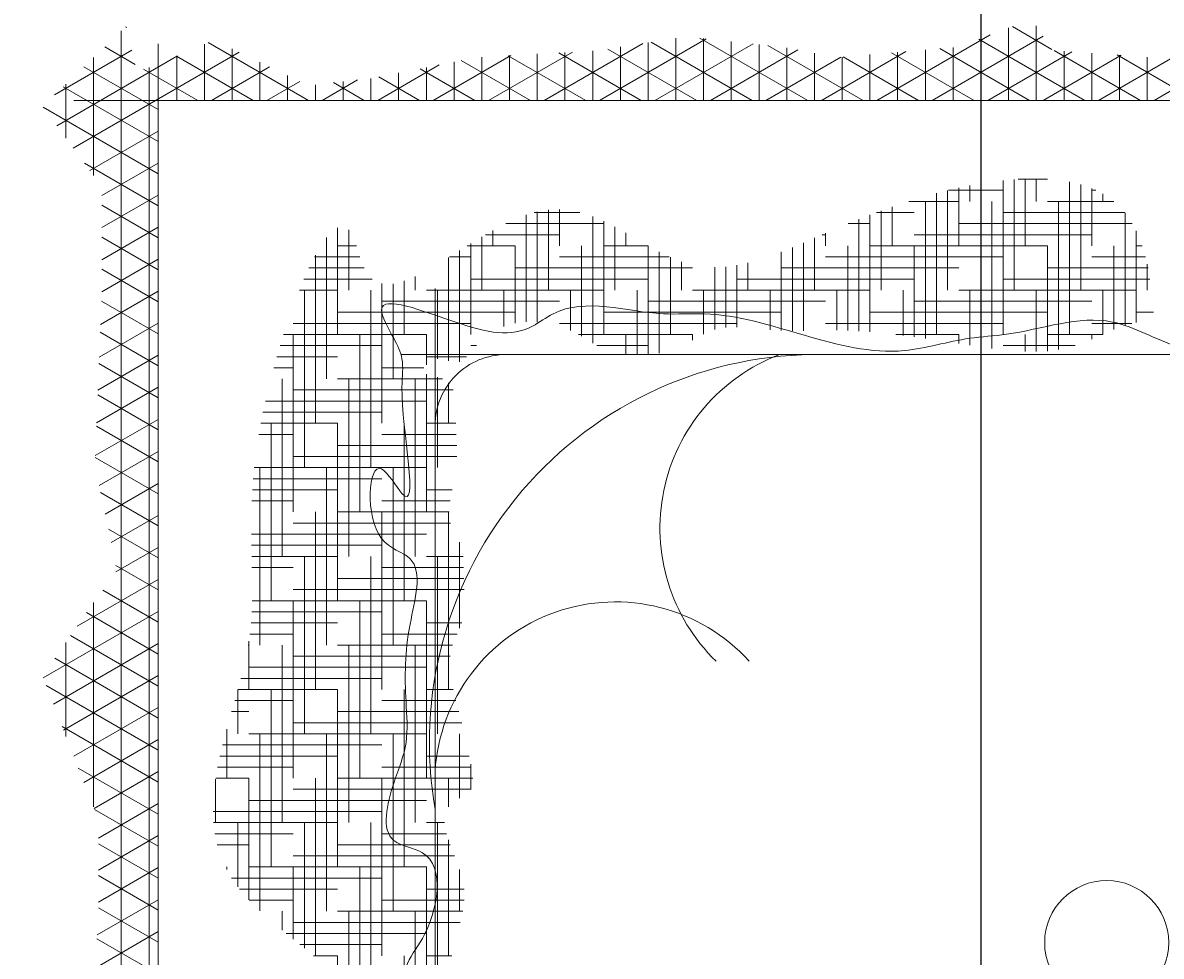
# Model space of a CAD drawing. Units: inches. Extents: x 3731 to 4318, y 1310 to 2388.
# Tile 12 of 57: x 3985 to 4038, y 1420 to 1463. Entities that reach past the tile are written whole.
import ezdxf

# ---------------------------------------------------------------- set-up
doc = ezdxf.new("R2010")
doc.units = ezdxf.units.IN
doc.layers.add('A-ANNO-DIMS', color=2, linetype='Continuous', lineweight=18)
doc.layers.add('A-FURN', color=8, linetype='Continuous', lineweight=13)
doc.styles.get("Standard").update_dxf_attribs({"font": 'arial.ttf'})
doc.dimstyles.get("Standard").update_dxf_attribs({"dimtxt": 0.18, "dimasz": 0.18, "dimexe": 0.18, "dimexo": 0.0625, "dimgap": 0.09, "dimtad": 0, "dimtih": 1, "dimtoh": 1, "dimdec": 4, "dimzin": 0, "dimdsep": 46, "dimtxsty": 'Standard', "dimcen": 0.09, "dimadec": 0, "dimazin": 0, "dimtfac": 1, "dimtdec": 4, "dimtofl": 0, "dimtmove": 0, "dimatfit": 3, "dimfxl": 1, "dimtolj": 1, "dimtzin": 0, "dimarcsym": 0})

# ---------------------------------------------------------------- blocks, each defined once
blk = doc.blocks.new('A$C200C7901')
for p, q in [((2.3121, 1.6596), (2.3121, 0.0201)), ((2, 0.2957), (2, 1.2957)), ((2.0224, 0.9977), (2.0224, 1.1977)), ((2.0224, 0.9977), (2.0224, 1.1977)), ((1.9974, 0.5977), (1.9974, 0.7977)), ((1.9974, 0.5977), (1.9974, 0.7977)), ((2.0724, 0.5977), (2.0724, 0.7977)), ((2.0724, 0.5977), (2.0724, 0.7977)), ((2.1474, 0.5977), (2.1474, 0.7977)), ((2.1474, 0.5977), (2.1474, 0.7977)), ((1.9849, 0.5477), (1.9849, 0.7477)), ((1.9849, 0.5477), (1.9849, 0.7477)), ((2.0599, 0.5477), (2.0599, 0.7477)), ((2.0599, 0.5477), (2.0599, 0.7477)), ((2.1349, 0.5477), (2.1349, 0.7477)), ((2.1349, 0.5477), (2.1349, 0.7477)), ((0.4061, 0.3703), (2.0386, 0.3703)), ((2.4073, 0.0839), (0.9625, 0.0839))]:
    blk.add_line(p, q)
at = {"linetype": 'ByBlock'}
for p, q in [((2.3224, 0.0468), (2.3224, 1.6627)), ((2.3224, 0.0468), (2.3224, 1.6627)), ((2.3537, 0.0056), (2.3537, 1.634)), ((2.3537, 0.0056), (2.3537, 1.634)), ((2.0349, 1.0477), (2.0349, 1.2477)), ((2.0349, 1.0477), (2.0349, 1.2477)), ((2.0099, 0.9477), (2.0099, 1.1477)), ((2.0099, 0.9477), (2.0099, 1.1477)), ((2.0849, 0.9477), (2.0849, 1.1477)), ((2.0849, 0.9477), (2.0849, 1.1477)), ((1.9974, 0.8977), (1.9974, 1.0977)), ((1.9974, 0.8977), (1.9974, 1.0977)), ((2.0724, 0.8977), (2.0724, 1.0977)), ((2.0724, 0.8977), (2.0724, 1.0977)), ((2.0974, 0.9977), (2.0974, 1.0909)), ((2.0974, 0.9977), (2.0974, 1.0909)), ((2.1099, 1.0477), (2.1099, 1.0729)), ((2.1099, 1.0477), (2.1099, 1.0729)), ((2.3121, 1.0686), (2.3813, 1.0286)), ((2.3121, 1.0686), (2.3813, 1.0286)), ((2.3121, 1.0206), (2.3851, 1.0628)), ((2.3121, 1.0206), (2.3851, 1.0628)), ((1.981, 1.0477), (2.0099, 1.0477)), ((1.981, 1.0477), (2.0099, 1.0477)), ((1.9849, 0.9171), (1.9849, 1.0477)), ((1.9849, 0.9171), (1.9849, 1.0477)), ((2.0599, 0.8477), (2.0599, 1.0477)), ((2.0599, 0.8477), (2.0599, 1.0477)), ((2.1099, 1.0477), (2.137, 1.0477)), ((2.1099, 1.0477), (2.137, 1.0477)), ((2.1349, 0.8477), (2.1349, 1.0477)), ((2.1349, 0.8477), (2.1349, 1.0477)), ((2.0599, 1.0352), (2.1523, 1.0352)), ((2.0599, 1.0352), (2.1523, 1.0352)), ((2.1474, 0.8977), (2.1474, 1.0391)), ((2.1474, 0.8977), (2.1474, 1.0391)), ((2.1599, 0.9477), (2.1599, 1.029)), ((2.1599, 0.9477), (2.1599, 1.029)), ((2.3121, 1.0325), (2.3795, 0.9936)), ((2.3121, 1.0325), (2.3795, 0.9936)), ((2.0099, 1.0227), (2.1678, 1.0227)), ((2.0099, 1.0227), (2.1678, 1.0227)), ((2.1724, 0.9977), (2.1724, 1.0189)), ((2.1724, 0.9977), (2.1724, 1.0189)), ((2.3121, 0.9846), (2.3809, 1.0242)), ((2.3121, 0.9846), (2.3809, 1.0242)), ((1.9718, 1.0102), (2.1599, 1.0102)), ((1.9718, 1.0102), (2.1599, 1.0102)), ((1.9688, 0.9977), (2.1099, 0.9977)), ((1.9688, 0.9977), (2.1099, 0.9977)), ((1.9724, 0.9504), (1.9724, 0.9977)), ((1.9724, 0.9504), (1.9724, 0.9977)), ((2.0474, 0.7977), (2.0474, 0.9977)), ((2.0474, 0.7977), (2.0474, 0.9977)), ((2.1224, 0.7977), (2.1224, 0.9977)), ((2.1224, 0.7977), (2.1224, 0.9977)), ((2.1974, 0.7977), (2.1974, 0.9972)), ((2.1974, 0.7977), (2.1974, 0.9972)), ((2.3121, 0.9964), (2.3795, 0.9575)), ((2.3121, 0.9964), (2.3795, 0.9575)), ((1.9671, 0.9852), (2.0599, 0.9852)), ((1.9671, 0.9852), (2.0599, 0.9852)), ((2.1599, 0.9852), (2.2095, 0.9852)), ((2.1599, 0.9852), (2.2095, 0.9852)), ((2.2099, 0.8477), (2.2099, 0.9848)), ((2.2099, 0.8477), (2.2099, 0.9848)), ((2.3121, 0.9485), (2.3795, 0.9874)), ((2.3121, 0.9485), (2.3795, 0.9874)), ((1.9672, 0.9727), (2.0099, 0.9727)), ((1.9672, 0.9727), (2.0099, 0.9727)), ((2.1099, 0.9727), (2.2204, 0.9727)), ((2.1099, 0.9727), (2.2204, 0.9727)), ((2.2224, 0.8977), (2.2224, 0.9702)), ((2.2224, 0.8977), (2.2224, 0.9702)), ((2.0599, 0.9602), (2.2294, 0.9602)), ((2.0599, 0.9602), (2.2294, 0.9602)), ((2.2349, 0.9477), (2.2349, 0.9506)), ((2.2349, 0.9477), (2.2349, 0.9506)), ((2.3121, 0.9603), (2.3795, 0.9215)), ((2.3121, 0.9603), (2.3795, 0.9215)), ((2.3121, 0.9124), (2.3795, 0.9513)), ((2.3121, 0.9124), (2.3795, 0.9513)), ((2.0099, 0.9477), (2.2099, 0.9477)), ((2.0099, 0.9477), (2.2099, 0.9477)), ((2.0349, 0.7477), (2.0349, 0.9477)), ((2.0349, 0.7477), (2.0349, 0.9477)), ((2.1099, 0.7477), (2.1099, 0.9477)), ((2.1099, 0.7477), (2.1099, 0.9477)), ((2.1849, 0.7477), (2.1849, 0.9477)), ((2.1849, 0.7477), (2.1849, 0.9477)), ((1.9781, 0.9352), (2.1599, 0.9352)), ((1.9781, 0.9352), (2.1599, 0.9352)), ((2.3121, 0.9243), (2.3838, 0.8829)), ((2.3121, 0.9243), (2.3838, 0.8829)), ((1.9829, 0.9227), (2.1099, 0.9227)), ((1.9829, 0.9227), (2.1099, 0.9227)), ((2.2099, 0.9227), (2.2455, 0.9227)), ((2.2099, 0.9227), (2.2455, 0.9227)), ((2.3121, 0.8763), (2.3795, 0.9152)), ((2.3121, 0.8763), (2.3795, 0.9152)), ((1.9871, 0.9102), (2.0599, 0.9102)), ((1.9871, 0.9102), (2.0599, 0.9102)), ((2.1599, 0.9102), (2.2481, 0.9102)), ((2.1599, 0.9102), (2.2481, 0.9102)), ((1.9894, 0.8977), (2.0099, 0.8977)), ((1.9894, 0.8977), (2.0099, 0.8977)), ((2.0224, 0.6977), (2.0224, 0.8977)), ((2.0224, 0.6977), (2.0224, 0.8977)), ((2.0974, 0.6977), (2.0974, 0.8977)), ((2.0974, 0.6977), (2.0974, 0.8977)), ((2.1099, 0.8977), (2.2496, 0.8977)), ((2.1099, 0.8977), (2.2496, 0.8977)), ((2.1724, 0.6977), (2.1724, 0.8977)), ((2.1724, 0.6977), (2.1724, 0.8977)), ((2.2474, 0.8489), (2.2474, 0.8977)), ((2.2474, 0.8489), (2.2474, 0.8977)), ((2.3121, 0.8882), (2.4022, 0.8362)), ((2.3121, 0.8882), (2.4022, 0.8362)), ((1.9849, 0.8477), (1.9849, 0.88)), ((1.9849, 0.8477), (1.9849, 0.88)), ((2.0099, 0.8727), (2.2099, 0.8727)), ((2.0099, 0.8727), (2.2099, 0.8727)), ((2.0599, 0.8852), (2.2501, 0.8852)), ((2.0599, 0.8852), (2.2501, 0.8852)), ((2.3121, 0.8402), (2.3842, 0.8818)), ((2.3121, 0.8402), (2.3842, 0.8818)), ((2.3849, 0.6497), (2.3849, 0.8801)), ((2.3849, 0.6497), (2.3849, 0.8801)), ((1.9599, 0.8317), (1.9599, 0.8604)), ((1.9599, 0.8317), (1.9599, 0.8604)), ((1.9599, 0.8602), (2.1599, 0.8602)), ((1.9599, 0.8602), (2.1599, 0.8602)), ((1.9724, 0.7977), (1.9724, 0.8703)), ((1.9724, 0.7977), (1.9724, 0.8703)), ((1.9574, 0.8477), (2.1099, 0.8477)), ((1.9574, 0.8477), (2.1099, 0.8477)), ((2.0099, 0.6477), (2.0099, 0.8477)), ((2.0099, 0.6477), (2.0099, 0.8477)), ((2.0849, 0.6477), (2.0849, 0.8477)), ((2.0849, 0.6477), (2.0849, 0.8477)), ((2.1599, 0.6477), (2.1599, 0.8477)), ((2.1599, 0.6477), (2.1599, 0.8477)), ((2.2099, 0.8477), (2.2472, 0.8477)), ((2.2099, 0.8477), (2.2472, 0.8477)), ((2.2349, 0.7923), (2.2349, 0.8477)), ((2.2349, 0.7923), (2.2349, 0.8477)), ((2.3121, 0.8041), (2.3958, 0.8524)), ((2.3121, 0.8041), (2.3958, 0.8524)), ((2.3121, 0.8521), (2.4205, 0.7895)), ((2.3121, 0.8521), (2.4205, 0.7895)), ((1.9593, 0.8352), (2.0599, 0.8352)), ((1.9593, 0.8352), (2.0599, 0.8352)), ((2.1599, 0.8352), (2.2451, 0.8352)), ((2.1599, 0.8352), (2.2451, 0.8352)), ((1.9615, 0.8227), (2.0099, 0.8227)), ((1.9615, 0.8227), (2.0099, 0.8227)), ((2.1099, 0.8227), (2.2425, 0.8227)), ((2.1099, 0.8227), (2.2425, 0.8227)), ((2.3121, 0.7681), (2.4073, 0.823)), ((2.3121, 0.7681), (2.4073, 0.823)), ((2.0599, 0.8102), (2.2396, 0.8102)), ((2.0599, 0.8102), (2.2396, 0.8102)), ((2.3121, 0.816), (2.4384, 0.7431)), ((2.3121, 0.816), (2.4384, 0.7431)), ((2.0099, 0.7977), (2.2099, 0.7977)), ((2.0099, 0.7977), (2.2099, 0.7977)), ((2.2224, 0.7483), (2.2224, 0.7977)), ((2.2224, 0.7483), (2.2224, 0.7977)), ((2.4162, 0.6946), (2.4162, 0.8006)), ((2.4162, 0.6946), (2.4162, 0.8006)), ((1.9699, 0.7852), (2.1599, 0.7852)), ((1.9699, 0.7852), (2.1599, 0.7852)), ((2.3121, 0.732), (2.4189, 0.7936)), ((2.3121, 0.732), (2.4189, 0.7936)), ((1.9734, 0.7727), (2.1099, 0.7727)), ((1.9734, 0.7727), (2.1099, 0.7727)), ((2.2099, 0.7727), (2.2294, 0.7727)), ((2.2099, 0.7727), (2.2294, 0.7727)), ((2.3121, 0.7799), (2.4287, 0.7126)), ((2.3121, 0.7799), (2.4287, 0.7126)), ((1.9767, 0.7602), (2.0599, 0.7602)), ((1.9767, 0.7602), (2.0599, 0.7602)), ((2.1599, 0.7602), (2.2258, 0.7602)), ((2.1599, 0.7602), (2.2258, 0.7602)), ((2.3121, 0.6959), (2.4303, 0.7641)), ((2.3121, 0.6959), (2.4303, 0.7641)), ((1.9797, 0.7477), (2.0099, 0.7477)), ((1.9797, 0.7477), (2.0099, 0.7477)), ((2.1099, 0.7477), (2.2222, 0.7477)), ((2.1099, 0.7477), (2.2222, 0.7477)), ((2.2099, 0.6933), (2.2099, 0.7477)), ((2.2099, 0.6933), (2.2099, 0.7477)), ((2.0599, 0.7352), (2.2188, 0.7352)), ((2.0599, 0.7352), (2.2188, 0.7352)), ((2.3121, 0.7438), (2.4108, 0.6869)), ((2.3121, 0.7438), (2.4108, 0.6869)), ((2.3121, 0.6598), (2.4417, 0.7346)), ((2.3121, 0.6598), (2.4417, 0.7346)), ((2.0099, 0.7227), (2.2099, 0.7227)), ((2.0099, 0.7227), (2.2099, 0.7227)), ((1.9831, 0.7102), (2.1599, 0.7102)), ((1.9831, 0.7102), (2.1599, 0.7102)), ((2.3121, 0.7078), (2.3929, 0.6611)), ((2.3121, 0.7078), (2.3929, 0.6611)), ((1.9804, 0.6977), (2.1099, 0.6977)), ((1.9804, 0.6977), (2.1099, 0.6977)), ((2.0474, 0.4977), (2.0474, 0.6977)), ((2.0474, 0.4977), (2.0474, 0.6977)), ((2.1224, 0.4977), (2.1224, 0.6977)), ((2.1224, 0.4977), (2.1224, 0.6977)), ((2.1974, 0.4977), (2.1974, 0.6977)), ((2.1974, 0.4977), (2.1974, 0.6977)), ((2.2099, 0.6977), (2.2106, 0.6977)), ((2.2099, 0.6977), (2.2106, 0.6977)), ((1.9753, 0.6852), (2.0599, 0.6852)), ((1.9753, 0.6852), (2.0599, 0.6852)), ((2.1599, 0.6852), (2.2088, 0.6852)), ((2.1599, 0.6852), (2.2088, 0.6852)), ((1.97, 0.6727), (2.0099, 0.6727)), ((1.97, 0.6727), (2.0099, 0.6727)), ((1.9724, 0.5818), (1.9724, 0.6786)), ((1.9724, 0.5818), (1.9724, 0.6786)), ((2.1099, 0.6727), (2.2075, 0.6727)), ((2.1099, 0.6727), (2.2075, 0.6727)), ((2.3121, 0.6237), (2.4036, 0.6765)), ((2.3121, 0.6237), (2.4036, 0.6765)), ((2.3121, 0.6717), (2.3744, 0.6357)), ((2.3121, 0.6717), (2.3744, 0.6357)), ((2.0599, 0.6602), (2.2067, 0.6602)), ((2.0599, 0.6602), (2.2067, 0.6602)), ((2.0099, 0.6477), (2.2062, 0.6477)), ((2.0099, 0.6477), (2.2062, 0.6477)), ((2.0349, 0.4477), (2.0349, 0.6477)), ((2.0349, 0.4477), (2.0349, 0.6477)), ((2.1099, 0.4477), (2.1099, 0.6477)), ((2.1099, 0.4477), (2.1099, 0.6477)), ((2.1849, 0.4477), (2.1849, 0.6477)), ((2.1849, 0.4477), (2.1849, 0.6477)), ((1.9673, 0.6352), (2.1599, 0.6352)), ((1.9673, 0.6352), (2.1599, 0.6352)), ((2.3121, 0.6356), (2.3598, 0.6081)), ((2.3121, 0.6356), (2.3598, 0.6081)), ((1.9678, 0.6227), (2.1099, 0.6227)), ((1.9678, 0.6227), (2.1099, 0.6227)), ((1.9679, 0.6102), (2.0599, 0.6102)), ((1.9679, 0.6102), (2.0599, 0.6102)), ((2.1599, 0.6102), (2.2064, 0.6102)), ((2.1599, 0.6102), (2.2064, 0.6102)), ((2.3121, 0.5876), (2.3598, 0.6151)), ((2.3121, 0.5876), (2.3598, 0.6151)), ((1.9685, 0.5977), (2.0099, 0.5977)), ((1.9685, 0.5977), (2.0099, 0.5977)), ((2.0224, 0.3977), (2.0224, 0.5977)), ((2.0224, 0.3977), (2.0224, 0.5977)), ((2.0974, 0.3977), (2.0974, 0.5977)), ((2.0974, 0.3977), (2.0974, 0.5977)), ((2.1099, 0.5977), (2.2066, 0.5977)), ((2.1099, 0.5977), (2.2066, 0.5977)), ((2.1724, 0.3977), (2.1724, 0.5977)), ((2.1724, 0.3977), (2.1724, 0.5977)), ((2.3121, 0.5995), (2.3682, 0.5671)), ((2.3121, 0.5995), (2.3682, 0.5671)), ((2.0599, 0.5852), (2.2069, 0.5852)), ((2.0599, 0.5852), (2.2069, 0.5852)), ((2.3121, 0.5515), (2.365, 0.5821)), ((2.3121, 0.5515), (2.365, 0.5821)), ((2.0099, 0.5727), (2.207, 0.5727)), ((2.0099, 0.5727), (2.207, 0.5727)), ((1.9827, 0.5602), (2.1599, 0.5602)), ((1.9827, 0.5602), (2.1599, 0.5602)), ((2.3121, 0.5634), (2.3771, 0.5259)), ((2.3121, 0.5634), (2.3771, 0.5259)), ((1.9842, 0.5477), (2.1099, 0.5477)), ((1.9842, 0.5477), (2.1099, 0.5477)), ((2.0099, 0.3923), (2.0099, 0.5477)), ((2.0099, 0.3923), (2.0099, 0.5477)), ((2.0849, 0.3477), (2.0849, 0.5477)), ((2.0849, 0.3477), (2.0849, 0.5477)), ((2.1599, 0.3477), (2.1599, 0.5477)), ((2.1599, 0.3477), (2.1599, 0.5477)), ((2.3121, 0.5155), (2.3719, 0.55)), ((2.3121, 0.5155), (2.3719, 0.55)), ((1.9831, 0.5352), (2.0599, 0.5352)), ((1.9831, 0.5352), (2.0599, 0.5352)), ((2.1599, 0.5352), (2.2065, 0.5352)), ((2.1599, 0.5352), (2.2065, 0.5352)), ((2.3121, 0.5273), (2.383, 0.4864)), ((2.3121, 0.5273), (2.383, 0.4864)), ((1.9807, 0.5227), (2.0099, 0.5227)), ((1.9807, 0.5227), (2.0099, 0.5227)), ((2.1099, 0.5227), (2.2058, 0.5227)), ((2.1099, 0.5227), (2.2058, 0.5227)), ((2.3121, 0.4794), (2.3788, 0.5179)), ((2.3121, 0.4794), (2.3788, 0.5179)), ((2.0599, 0.5102), (2.2049, 0.5102)), ((2.0599, 0.5102), (2.2049, 0.5102)), ((1.9974, 0.3957), (1.9974, 0.4977)), ((1.9974, 0.3957), (1.9974, 0.4977)), ((2.0099, 0.4977), (2.2038, 0.4977)), ((2.0099, 0.4977), (2.2038, 0.4977)), ((2.0724, 0.2977), (2.0724, 0.4977)), ((2.0724, 0.2977), (2.0724, 0.4977)), ((2.1474, 0.2977), (2.1474, 0.4977)), ((2.1474, 0.2977), (2.1474, 0.4977)), ((2.3121, 0.4912), (2.3817, 0.4511)), ((2.3121, 0.4912), (2.3817, 0.4511)), ((1.9755, 0.4852), (2.1599, 0.4852)), ((1.9755, 0.4852), (2.1599, 0.4852)), ((2.3121, 0.4433), (2.383, 0.4842)), ((2.3121, 0.4433), (2.383, 0.4842)), ((1.9757, 0.4727), (2.1099, 0.4727)), ((1.9757, 0.4727), (2.1099, 0.4727)), ((1.9762, 0.4602), (2.0599, 0.4602)), ((1.9762, 0.4602), (2.0599, 0.4602)), ((2.1599, 0.4602), (2.1987, 0.4602)), ((2.1599, 0.4602), (2.1987, 0.4602)), ((2.3121, 0.4552), (2.3803, 0.4158)), ((2.3121, 0.4552), (2.3803, 0.4158)), ((1.9768, 0.4477), (2.0099, 0.4477)), ((1.9768, 0.4477), (2.0099, 0.4477)), ((1.9849, 0.402), (1.9849, 0.4477)), ((1.9849, 0.402), (1.9849, 0.4477)), ((2.0599, 0.2903), (2.0599, 0.4477)), ((2.0599, 0.2903), (2.0599, 0.4477)), ((2.1099, 0.4477), (2.1965, 0.4477)), ((2.1099, 0.4477), (2.1965, 0.4477)), ((2.1349, 0.2582), (2.1349, 0.4477)), ((2.1349, 0.2582), (2.1349, 0.4477)), ((2.3121, 0.4072), (2.3815, 0.4473)), ((2.3121, 0.4072), (2.3815, 0.4473)), ((2.0599, 0.4352), (2.194, 0.4352)), ((2.0599, 0.4352), (2.194, 0.4352)), ((2.0099, 0.4227), (2.1913, 0.4227)), ((2.0099, 0.4227), (2.1913, 0.4227)), ((2.3121, 0.4191), (2.3789, 0.3805)), ((2.3121, 0.4191), (2.3789, 0.3805)), ((1.9797, 0.4102), (2.1599, 0.4102)), ((1.9797, 0.4102), (2.1599, 0.4102)), ((2.3121, 0.3711), (2.3801, 0.4103)), ((2.3121, 0.3711), (2.3801, 0.4103)), ((1.9915, 0.3977), (2.1099, 0.3977)), ((1.9915, 0.3977), (2.1099, 0.3977)), ((2.0127, 0.3852), (2.0599, 0.3852)), ((2.0127, 0.3852), (2.0599, 0.3852)), ((2.0474, 0.2905), (2.0474, 0.3977)), ((2.0474, 0.2905), (2.0474, 0.3977)), ((2.1224, 0.2385), (2.1224, 0.3977)), ((2.1224, 0.2385), (2.1224, 0.3977)), ((2.1599, 0.3852), (2.1819, 0.3852)), ((2.1599, 0.3852), (2.1819, 0.3852)), ((1.9648, 0.3727), (2.0099, 0.3727)), ((1.9648, 0.3727), (2.0099, 0.3727)), ((1.9724, 0.253), (1.9724, 0.3785)), ((1.9724, 0.253), (1.9724, 0.3785)), ((1.9849, 0.2609), (1.9849, 0.3774)), ((1.9849, 0.2609), (1.9849, 0.3774)), ((1.9974, 0.2977), (1.9974, 0.3753)), ((1.9974, 0.2977), (1.9974, 0.3753)), ((2.0099, 0.3477), (2.0099, 0.382)), ((2.0099, 0.3477), (2.0099, 0.382)), ((2.1099, 0.3727), (2.1784, 0.3727)), ((2.1099, 0.3727), (2.1784, 0.3727)), ((2.3121, 0.383), (2.3775, 0.3452)), ((2.3121, 0.383), (2.3775, 0.3452)), ((2.3121, 0.335), (2.3786, 0.3734)), ((2.3121, 0.335), (2.3786, 0.3734)), ((1.2785, 0.3602), (1.3599, 0.3602)), ((1.2785, 0.3602), (1.3599, 0.3602)), ((1.2974, 0.1977), (1.2974, 0.3647)), ((1.2974, 0.1977), (1.2974, 0.3647)), ((1.3099, 0.2477), (1.3099, 0.3663)), ((1.3099, 0.2477), (1.3099, 0.3663)), ((1.3224, 0.2977), (1.3224, 0.3669)), ((1.3224, 0.2977), (1.3224, 0.3669)), ((1.3349, 0.3477), (1.3349, 0.3668)), ((1.3349, 0.3477), (1.3349, 0.3668)), ((1.3724, 0.1977), (1.3724, 0.3634)), ((1.3724, 0.1977), (1.3724, 0.3634)), ((1.3849, 0.2477), (1.3849, 0.3616)), ((1.3849, 0.2477), (1.3849, 0.3616)), ((1.3974, 0.2977), (1.3974, 0.3597)), ((1.3974, 0.2977), (1.3974, 0.3597)), ((1.7474, 0.2546), (1.7474, 0.3689)), ((1.7474, 0.2546), (1.7474, 0.3689)), ((1.7599, 0.2477), (1.7599, 0.3703)), ((1.7599, 0.2477), (1.7599, 0.3703)), ((1.7599, 0.3602), (1.8177, 0.3602)), ((1.7599, 0.3602), (1.8177, 0.3602)), ((1.7724, 0.2977), (1.7724, 0.3703)), ((1.7724, 0.2977), (1.7724, 0.3703)), ((1.7849, 0.3477), (1.7849, 0.3703)), ((1.7849, 0.3477), (1.7849, 0.3703)), ((1.9532, 0.3602), (1.9599, 0.3602)), ((1.9532, 0.3602), (1.9599, 0.3602)), ((2.0599, 0.3602), (2.1747, 0.3602)), ((2.0599, 0.3602), (2.1747, 0.3602)), ((1.2474, 0.2977), (1.2474, 0.3476)), ((1.2474, 0.2977), (1.2474, 0.3476)), ((1.2475, 0.3477), (1.3099, 0.3477)), ((1.2475, 0.3477), (1.3099, 0.3477)), ((1.2599, 0.3477), (1.2599, 0.3531)), ((1.2599, 0.3477), (1.2599, 0.3531)), ((1.2849, 0.1758), (1.2849, 0.3477)), ((1.2849, 0.1758), (1.2849, 0.3477)), ((1.3599, 0.1741), (1.3599, 0.3477)), ((1.3599, 0.1741), (1.3599, 0.3477)), ((1.4099, 0.3477), (1.4099, 0.3578)), ((1.4099, 0.3477), (1.4099, 0.3578)), ((1.4099, 0.3477), (1.4806, 0.3477)), ((1.4099, 0.3477), (1.4806, 0.3477)), ((1.4349, 0.1886), (1.4349, 0.3477)), ((1.4349, 0.1886), (1.4349, 0.3477)), ((1.4474, 0.1977), (1.4474, 0.3521)), ((1.4474, 0.1977), (1.4474, 0.3521)), ((1.4599, 0.2477), (1.4599, 0.3504)), ((1.4599, 0.2477), (1.4599, 0.3504)), ((1.4724, 0.2977), (1.4724, 0.3487)), ((1.4724, 0.2977), (1.4724, 0.3487)), ((1.6974, 0.2977), (1.6974, 0.3472)), ((1.6974, 0.2977), (1.6974, 0.3472)), ((1.7099, 0.3477), (1.7099, 0.3539)), ((1.7099, 0.3477), (1.7099, 0.3539)), ((1.7099, 0.3477), (1.8383, 0.3477)), ((1.7099, 0.3477), (1.8383, 0.3477)), ((1.7349, 0.2607), (1.7349, 0.3477)), ((1.7349, 0.2607), (1.7349, 0.3477)), ((1.8099, 0.2201), (1.8099, 0.3477)), ((1.8099, 0.2201), (1.8099, 0.3477)), ((1.8224, 0.2148), (1.8224, 0.3575)), ((1.8224, 0.2148), (1.8224, 0.3575)), ((1.8349, 0.2477), (1.8349, 0.3497)), ((1.8349, 0.2477), (1.8349, 0.3497)), ((1.9599, 0.2452), (1.9599, 0.3477)), ((1.9599, 0.2452), (1.9599, 0.3477)), ((2.0099, 0.3477), (2.1708, 0.3477)), ((2.0099, 0.3477), (2.1708, 0.3477)), ((2.0349, 0.2874), (2.0349, 0.3477)), ((2.0349, 0.2874), (2.0349, 0.3477)), ((2.1099, 0.2274), (2.1099, 0.3477)), ((2.1099, 0.2274), (2.1099, 0.3477)), ((2.3121, 0.3469), (2.3761, 0.31)), ((2.3121, 0.3469), (2.3761, 0.31)), ((1.2099, 0.2308), (1.2099, 0.334)), ((1.2099, 0.2308), (1.2099, 0.334)), ((1.2148, 0.3352), (1.2599, 0.3352)), ((1.2148, 0.3352), (1.2599, 0.3352)), ((1.2224, 0.2106), (1.2224, 0.3375)), ((1.2224, 0.2106), (1.2224, 0.3375)), ((1.2349, 0.2477), (1.2349, 0.3422)), ((1.2349, 0.2477), (1.2349, 0.3422)), ((1.3599, 0.3352), (1.5599, 0.3352)), ((1.3599, 0.3352), (1.5599, 0.3352)), ((1.5099, 0.2129), (1.5099, 0.3447)), ((1.5099, 0.2129), (1.5099, 0.3447)), ((1.5224, 0.2177), (1.5224, 0.3438)), ((1.5224, 0.2177), (1.5224, 0.3438)), ((1.5349, 0.2477), (1.5349, 0.3431)), ((1.5349, 0.2477), (1.5349, 0.3431)), ((1.5474, 0.2977), (1.5474, 0.3428)), ((1.5474, 0.2977), (1.5474, 0.3428)), ((1.5849, 0.2443), (1.5849, 0.3434)), ((1.5849, 0.2443), (1.5849, 0.3434)), ((1.5974, 0.2496), (1.5974, 0.3435)), ((1.5974, 0.2496), (1.5974, 0.3435)), ((1.6099, 0.2546), (1.6099, 0.3432)), ((1.6099, 0.2546), (1.6099, 0.3432)), ((1.6224, 0.2977), (1.6224, 0.3424)), ((1.6224, 0.2977), (1.6224, 0.3424)), ((1.6599, 0.2695), (1.6599, 0.3394)), ((1.6599, 0.2695), (1.6599, 0.3394)), ((1.6599, 0.3352), (1.8599, 0.3352)), ((1.6599, 0.3352), (1.8599, 0.3352)), ((1.6724, 0.2713), (1.6724, 0.3398)), ((1.6724, 0.2713), (1.6724, 0.3398)), ((1.6849, 0.272), (1.6849, 0.3422)), ((1.6849, 0.272), (1.6849, 0.3422)), ((1.8474, 0.2977), (1.8474, 0.3432)), ((1.8474, 0.2977), (1.8474, 0.3432)), ((1.8849, 0.2093), (1.8849, 0.3337)), ((1.8849, 0.2093), (1.8849, 0.3337)), ((1.9099, 0.2477), (1.9099, 0.3349)), ((1.9099, 0.2477), (1.9099, 0.3349)), ((1.9224, 0.2977), (1.9224, 0.3385)), ((1.9224, 0.2977), (1.9224, 0.3385)), ((1.9599, 0.3352), (2.1599, 0.3352)), ((1.9599, 0.3352), (2.1599, 0.3352)), ((2.3121, 0.299), (2.3772, 0.3365)), ((2.3121, 0.299), (2.3772, 0.3365)), ((1.1904, 0.3227), (1.2099, 0.3227)), ((1.1904, 0.3227), (1.2099, 0.3227)), ((1.3099, 0.3227), (1.5099, 0.3227)), ((1.3099, 0.3227), (1.5099, 0.3227)), ((1.6099, 0.3227), (1.8099, 0.3227)), ((1.6099, 0.3227), (1.8099, 0.3227)), ((1.8974, 0.2129), (1.8974, 0.3335)), ((1.8974, 0.2129), (1.8974, 0.3335)), ((1.9099, 0.3227), (2.1099, 0.3227)), ((1.9099, 0.3227), (2.1099, 0.3227)), ((1.2599, 0.3102), (1.4599, 0.3102)), ((1.2599, 0.3102), (1.4599, 0.3102)), ((1.5599, 0.3102), (1.7599, 0.3102)), ((1.5599, 0.3102), (1.7599, 0.3102)), ((1.8599, 0.3102), (2.0599, 0.3102)), ((1.8599, 0.3102), (2.0599, 0.3102)), ((2.3121, 0.3108), (2.3755, 0.2742)), ((2.3121, 0.3108), (2.3755, 0.2742)), ((1.1974, 0.2683), (1.1974, 0.2977)), ((1.1974, 0.2683), (1.1974, 0.2977)), ((1.2099, 0.2977), (1.4099, 0.2977)), ((1.2099, 0.2977), (1.4099, 0.2977)), ((1.2724, 0.1788), (1.2724, 0.2977)), ((1.2724, 0.1788), (1.2724, 0.2977)), ((1.3474, 0.173), (1.3474, 0.2977)), ((1.3474, 0.173), (1.3474, 0.2977)), ((1.4224, 0.1854), (1.4224, 0.2977)), ((1.4224, 0.1854), (1.4224, 0.2977)), ((1.4974, 0.2083), (1.4974, 0.2977)), ((1.4974, 0.2083), (1.4974, 0.2977)), ((1.5099, 0.2977), (1.7099, 0.2977)), ((1.5099, 0.2977), (1.7099, 0.2977)), ((1.5724, 0.2389), (1.5724, 0.2977)), ((1.5724, 0.2389), (1.5724, 0.2977)), ((1.6474, 0.2668), (1.6474, 0.2977)), ((1.6474, 0.2668), (1.6474, 0.2977)), ((1.7224, 0.2658), (1.7224, 0.2977)), ((1.7224, 0.2658), (1.7224, 0.2977)), ((1.7974, 0.2263), (1.7974, 0.2977)), ((1.7974, 0.2263), (1.7974, 0.2977)), ((1.8099, 0.2977), (2.0099, 0.2977)), ((1.8099, 0.2977), (2.0099, 0.2977)), ((1.8724, 0.2072), (1.8724, 0.2977)), ((1.8724, 0.2072), (1.8724, 0.2977)), ((1.9474, 0.2376), (1.9474, 0.2977)), ((1.9474, 0.2376), (1.9474, 0.2977)), ((2.0224, 0.2822), (2.0224, 0.2977)), ((2.0224, 0.2822), (2.0224, 0.2977)), ((2.0974, 0.2299), (2.0974, 0.2977)), ((2.0974, 0.2299), (2.0974, 0.2977)), ((2.1099, 0.2977), (2.153, 0.2977)), ((2.1099, 0.2977), (2.153, 0.2977)), ((2.3121, 0.2629), (2.3757, 0.2996)), ((2.3121, 0.2629), (2.3757, 0.2996)), ((1.1943, 0.2852), (1.3599, 0.2852)), ((1.1943, 0.2852), (1.3599, 0.2852)), ((1.4599, 0.2852), (1.6599, 0.2852)), ((1.4599, 0.2852), (1.6599, 0.2852)), ((1.7599, 0.2852), (1.9599, 0.2852)), ((1.7599, 0.2852), (1.9599, 0.2852)), ((2.0708, 0.2852), (2.1478, 0.2852)), ((2.0708, 0.2852), (2.1478, 0.2852)), ((1.1965, 0.2727), (1.3099, 0.2727)), ((1.1965, 0.2727), (1.3099, 0.2727)), ((1.4099, 0.2727), (1.6099, 0.2727)), ((1.4099, 0.2727), (1.6099, 0.2727)), ((1.7099, 0.2727), (1.9099, 0.2727)), ((1.7099, 0.2727), (1.9099, 0.2727)), ((2.08, 0.2727), (2.1422, 0.2727)), ((2.08, 0.2727), (2.1422, 0.2727)), ((2.3121, 0.2747), (2.3755, 0.2381)), ((2.3121, 0.2747), (2.3755, 0.2381)), ((1.1994, 0.2602), (1.2599, 0.2602)), ((1.1994, 0.2602), (1.2599, 0.2602)), ((1.3599, 0.2602), (1.5599, 0.2602)), ((1.3599, 0.2602), (1.5599, 0.2602)), ((1.7361, 0.2602), (1.8599, 0.2602)), ((1.7361, 0.2602), (1.8599, 0.2602)), ((1.9599, 0.2602), (1.9838, 0.2602)), ((1.9599, 0.2602), (1.9838, 0.2602)), ((2.0848, 0.2602), (2.1359, 0.2602)), ((2.0848, 0.2602), (2.1359, 0.2602)), ((2.3121, 0.2268), (2.3755, 0.2634)), ((2.3121, 0.2268), (2.3755, 0.2634)), ((1.2031, 0.2477), (1.2099, 0.2477)), ((1.2031, 0.2477), (1.2099, 0.2477)), ((1.2599, 0.1831), (1.2599, 0.2477)), ((1.2599, 0.1831), (1.2599, 0.2477)), ((1.3099, 0.2477), (1.5099, 0.2477)), ((1.3099, 0.2477), (1.5099, 0.2477)), ((1.3349, 0.1723), (1.3349, 0.2477)), ((1.3349, 0.1723), (1.3349, 0.2477)), ((1.4099, 0.1825), (1.4099, 0.2477)), ((1.4099, 0.1825), (1.4099, 0.2477)), ((1.4849, 0.2039), (1.4849, 0.2477)), ((1.4849, 0.2039), (1.4849, 0.2477)), ((1.5599, 0.2335), (1.5599, 0.2477)), ((1.5599, 0.2335), (1.5599, 0.2477)), ((1.7599, 0.2477), (1.8099, 0.2477)), ((1.7599, 0.2477), (1.8099, 0.2477)), ((1.7849, 0.2332), (1.7849, 0.2477)), ((1.7849, 0.2332), (1.7849, 0.2477)), ((1.8599, 0.2068), (1.8599, 0.2477)), ((1.8599, 0.2068), (1.8599, 0.2477)), ((1.9099, 0.2477), (1.9639, 0.2477)), ((1.9099, 0.2477), (1.9639, 0.2477)), ((1.9349, 0.2304), (1.9349, 0.2477)), ((1.9349, 0.2304), (1.9349, 0.2477)), ((2.0888, 0.2477), (2.1099, 0.2477)), ((2.0888, 0.2477), (2.1099, 0.2477)), ((1.2599, 0.2352), (1.4599, 0.2352)), ((1.2599, 0.2352), (1.4599, 0.2352)), ((1.5599, 0.2352), (1.5638, 0.2352)), ((1.5599, 0.2352), (1.5638, 0.2352)), ((1.8599, 0.2352), (1.9433, 0.2352)), ((1.8599, 0.2352), (1.9433, 0.2352)), ((2.3121, 0.2387), (2.3755, 0.202)), ((2.3121, 0.2387), (2.3755, 0.202)), ((1.2142, 0.2227), (1.4099, 0.2227)), ((1.2142, 0.2227), (1.4099, 0.2227)), ((1.5099, 0.2227), (1.5346, 0.2227)), ((1.5099, 0.2227), (1.5346, 0.2227)), ((1.8099, 0.2227), (1.9203, 0.2227)), ((1.8099, 0.2227), (1.9203, 0.2227)), ((2.3121, 0.1907), (2.3755, 0.2273)), ((2.3121, 0.1907), (2.3755, 0.2273)), ((1.2227, 0.2102), (1.3599, 0.2102)), ((1.2227, 0.2102), (1.3599, 0.2102)), ((1.4599, 0.2102), (1.5027, 0.2102)), ((1.4599, 0.2102), (1.5027, 0.2102)), ((1.8368, 0.2102), (1.8884, 0.2102)), ((1.8368, 0.2102), (1.8884, 0.2102)), ((1.2351, 0.1977), (1.3099, 0.1977)), ((1.2351, 0.1977), (1.3099, 0.1977)), ((1.2474, 0.1892), (1.2474, 0.1977)), ((1.2474, 0.1892), (1.2474, 0.1977)), ((1.3224, 0.1722), (1.3224, 0.1977)), ((1.3224, 0.1722), (1.3224, 0.1977)), ((1.3974, 0.1799), (1.3974, 0.1977)), ((1.3974, 0.1799), (1.3974, 0.1977)), ((1.4099, 0.1977), (1.4662, 0.1977)), ((1.4099, 0.1977), (1.4662, 0.1977)), ((2.3121, 0.2026), (2.3953, 0.1545)), ((2.3121, 0.2026), (2.3953, 0.1545)), ((1.2552, 0.1852), (1.2599, 0.1852)), ((1.2552, 0.1852), (1.2599, 0.1852)), ((1.3599, 0.1852), (1.4215, 0.1852)), ((1.3599, 0.1852), (1.4215, 0.1852)), ((2.3121, 0.1546), (2.3755, 0.1912)), ((2.3121, 0.1546), (2.3755, 0.1912)), ((1.3099, 0.1727), (1.3428, 0.1727)), ((1.3099, 0.1727), (1.3428, 0.1727)), ((2.3849, 0.0355), (2.3849, 0.1686)), ((2.3849, 0.0355), (2.3849, 0.1686)), ((2.3121, 0.1665), (2.4419, 0.0916)), ((2.3121, 0.1665), (2.4419, 0.0916)), ((2.3121, 0.1185), (2.3891, 0.163)), ((2.3121, 0.1185), (2.3891, 0.163)), ((2.2208, 0.0297), (2.4078, 0.1377)), ((2.2208, 0.0297), (2.4078, 0.1377)), ((2.3121, 0.1304), (2.4193, 0.0685)), ((2.3121, 0.1304), (2.4193, 0.0685)), ((2.4162, 0.0655), (2.4162, 0.1264)), ((2.4162, 0.0655), (2.4162, 0.1264)), ((2.2903, 0.0337), (2.4265, 0.1124)), ((2.2903, 0.0337), (2.4265, 0.1124)), ((2.3121, 0.0943), (2.3958, 0.046)), ((2.3121, 0.0943), (2.3958, 0.046)), ((1.0891, 0.0259), (1.1897, 0.0839)), ((1.0891, 0.0259), (1.1897, 0.0839)), ((1.1426, 0.0839), (1.2313, 0.0327)), ((1.1426, 0.0839), (1.2313, 0.0327)), ((1.1642, 0.0331), (1.2522, 0.0839)), ((1.1642, 0.0331), (1.2522, 0.0839)), ((1.1974, 0.0351), (1.1974, 0.0839)), ((1.1974, 0.0351), (1.1974, 0.0839)), ((1.2051, 0.0839), (1.3023, 0.0278)), ((1.2051, 0.0839), (1.3023, 0.0278)), ((1.2266, 0.033), (1.3147, 0.0839)), ((1.2266, 0.033), (1.3147, 0.0839)), ((1.2287, 0.0329), (1.2287, 0.0839)), ((1.2287, 0.0329), (1.2287, 0.0839)), ((1.2599, 0.0308), (1.2599, 0.0839)), ((1.2599, 0.0308), (1.2599, 0.0839)), ((1.2676, 0.0839), (1.3871, 0.015)), ((1.2676, 0.0839), (1.3871, 0.015)), ((1.2824, 0.0292), (1.3772, 0.0839)), ((1.2824, 0.0292), (1.3772, 0.0839)), ((1.2912, 0.0286), (1.2912, 0.0839)), ((1.2912, 0.0286), (1.2912, 0.0839)), ((1.3146, 0.0117), (1.4397, 0.0839)), ((1.3146, 0.0117), (1.4397, 0.0839)), ((1.3224, 0), (1.3224, 0.0839)), ((1.3224, 0), (1.3224, 0.0839)), ((1.3301, 0.0839), (1.4312, 0.0256)), ((1.3301, 0.0839), (1.4312, 0.0256)), ((1.3537, 0.0022), (1.3537, 0.0839)), ((1.3537, 0.0022), (1.3537, 0.0839)), ((1.3743, 0.0101), (1.5022, 0.0839)), ((1.3743, 0.0101), (1.5022, 0.0839)), ((1.3849, 0.0141), (1.3849, 0.0839)), ((1.3849, 0.0141), (1.3849, 0.0839)), ((1.3926, 0.0839), (1.4856, 0.0302)), ((1.3926, 0.0839), (1.4856, 0.0302)), ((1.4162, 0.0243), (1.4162, 0.0839)), ((1.4162, 0.0243), (1.4162, 0.0839)), ((1.4474, 0.027), (1.4474, 0.0839)), ((1.4474, 0.027), (1.4474, 0.0839)), ((1.4551, 0.0839), (1.54, 0.0349)), ((1.4551, 0.0839), (1.54, 0.0349)), ((1.4693, 0.0288), (1.5647, 0.0839)), ((1.4693, 0.0288), (1.5647, 0.0839)), ((1.4787, 0.0296), (1.4787, 0.0839)), ((1.4787, 0.0296), (1.4787, 0.0839)), ((1.5099, 0.0323), (1.5099, 0.0839)), ((1.5099, 0.0323), (1.5099, 0.0839)), ((1.5176, 0.0839), (1.6251, 0.0219)), ((1.5176, 0.0839), (1.6251, 0.0219)), ((1.5412, 0.035), (1.5412, 0.0839)), ((1.5412, 0.035), (1.5412, 0.0839)), ((1.5427, 0.0351), (1.6272, 0.0839)), ((1.5427, 0.0351), (1.6272, 0.0839)), ((1.5724, 0.0308), (1.5724, 0.0839)), ((1.5724, 0.0308), (1.5724, 0.0839)), ((1.5801, 0.0839), (1.7018, 0.0137)), ((1.5801, 0.0839), (1.7018, 0.0137)), ((1.5911, 0.027), (1.6897, 0.0839)), ((1.5911, 0.027), (1.6897, 0.0839)), ((1.6037, 0.0245), (1.6037, 0.0839)), ((1.6037, 0.0245), (1.6037, 0.0839)), ((1.6349, 0.0208), (1.6349, 0.0839)), ((1.6349, 0.0208), (1.6349, 0.0839)), ((1.6416, 0.0201), (1.7522, 0.0839)), ((1.6416, 0.0201), (1.7522, 0.0839)), ((1.6426, 0.0839), (1.7565, 0.0182)), ((1.6426, 0.0839), (1.7565, 0.0182)), ((1.6662, 0.0175), (1.6662, 0.0839)), ((1.6662, 0.0175), (1.6662, 0.0839)), ((1.6944, 0.0145), (1.8147, 0.0839)), ((1.6944, 0.0145), (1.8147, 0.0839)), ((1.6974, 0.0141), (1.6974, 0.0839)), ((1.6974, 0.0141), (1.6974, 0.0839)), ((1.7051, 0.0839), (1.8054, 0.026)), ((1.7051, 0.0839), (1.8054, 0.026)), ((1.7287, 0.0137), (1.7287, 0.0839)), ((1.7287, 0.0137), (1.7287, 0.0839)), ((1.7599, 0.0187), (1.7599, 0.0839)), ((1.7599, 0.0187), (1.7599, 0.0839)), ((1.7659, 0.0197), (1.8772, 0.0839)), ((1.7659, 0.0197), (1.8772, 0.0839)), ((1.7676, 0.0839), (1.8606, 0.0303)), ((1.7676, 0.0839), (1.8606, 0.0303)), ((1.7912, 0.0237), (1.7912, 0.0839)), ((1.7912, 0.0237), (1.7912, 0.0839)), ((1.8224, 0.0281), (1.8224, 0.0839)), ((1.8224, 0.0281), (1.8224, 0.0839)), ((1.8301, 0.0839), (1.9175, 0.0335)), ((1.8301, 0.0839), (1.9175, 0.0335)), ((1.8452, 0.0294), (1.9397, 0.0839)), ((1.8452, 0.0294), (1.9397, 0.0839)), ((1.8537, 0.0299), (1.8537, 0.0839)), ((1.8537, 0.0299), (1.8537, 0.0839)), ((1.8849, 0.0316), (1.8849, 0.0839)), ((1.8849, 0.0316), (1.8849, 0.0839)), ((1.8926, 0.0839), (1.9706, 0.0389)), ((1.8926, 0.0839), (1.9706, 0.0389)), ((1.9146, 0.0333), (2.0022, 0.0839)), ((1.9146, 0.0333), (2.0022, 0.0839)), ((1.9162, 0.0334), (1.9162, 0.0839)), ((1.9162, 0.0334), (1.9162, 0.0839)), ((1.9474, 0.0352), (1.9474, 0.0839)), ((1.9474, 0.0352), (1.9474, 0.0839)), ((1.9551, 0.0839), (2.017, 0.0482)), ((1.9551, 0.0839), (2.017, 0.0482)), ((1.9787, 0.0405), (1.9787, 0.0839)), ((1.9787, 0.0405), (1.9787, 0.0839)), ((1.9953, 0.0438), (2.0647, 0.0839)), ((1.9953, 0.0438), (2.0647, 0.0839)), ((2.0099, 0.0468), (2.0099, 0.0839)), ((2.0099, 0.0468), (2.0099, 0.0839)), ((2.0176, 0.0839), (2.0634, 0.0575)), ((2.0176, 0.0839), (2.0634, 0.0575)), ((2.0412, 0.053), (2.0412, 0.0839)), ((2.0412, 0.053), (2.0412, 0.0839)), ((2.0724, 0.0592), (2.0724, 0.0839)), ((2.0724, 0.0592), (2.0724, 0.0839)), ((2.0801, 0.0839), (2.1147, 0.0639)), ((2.0801, 0.0839), (2.1147, 0.0639)), ((2.0873, 0.0609), (2.1272, 0.0839)), ((2.0873, 0.0609), (2.1272, 0.0839)), ((2.1037, 0.0627), (2.1037, 0.0839)), ((2.1037, 0.0627), (2.1037, 0.0839)), ((2.1349, 0.0662), (2.1349, 0.0839)), ((2.1349, 0.0662), (2.1349, 0.0839)), ((2.1426, 0.0839), (2.2557, 0.0186)), ((2.1426, 0.0839), (2.2557, 0.0186)), ((2.1526, 0.0625), (2.1897, 0.0839)), ((2.1526, 0.0625), (2.1897, 0.0839)), ((2.1662, 0.056), (2.1662, 0.0839)), ((2.1662, 0.056), (2.1662, 0.0839)), ((2.1867, 0.0461), (2.2522, 0.0839)), ((2.1867, 0.0461), (2.2522, 0.0839)), ((2.1974, 0.041), (2.1974, 0.0839)), ((2.1974, 0.041), (2.1974, 0.0839)), ((2.2051, 0.0839), (2.2913, 0.0342)), ((2.2051, 0.0839), (2.2913, 0.0342)), ((2.2287, 0.0259), (2.2287, 0.0839)), ((2.2287, 0.0259), (2.2287, 0.0839)), ((2.2599, 0.0205), (2.2599, 0.0839)), ((2.2599, 0.0205), (2.2599, 0.0839)), ((2.2676, 0.0839), (2.3285, 0.0488)), ((2.2676, 0.0839), (2.3285, 0.0488)), ((2.2912, 0.0341), (2.2912, 0.0839)), ((2.2912, 0.0341), (2.2912, 0.0839)), ((2.3417, 0.0273), (2.429, 0.0777)), ((2.3417, 0.0273), (2.429, 0.0777)), ((2.338, 0.0433), (2.3723, 0.0235)), ((2.338, 0.0433), (2.3723, 0.0235)), ((1.3048, 0.0264), (1.3494, 0.0006)), ((1.3048, 0.0264), (1.3494, 0.0006)), ((2.3476, 0.0017), (2.3488, 0.001)), ((2.3476, 0.0017), (2.3488, 0.001))]:
    blk.add_line(p, q, dxfattribs=at)
blk.add_circle((1.2431, 1.0329), 0.0699)
for centre, radius, start, end in [((1.5693, 0.8075), 0.4372, 269.0679, 9.9322), ((1.7969, 0.8525), 0.2035, 222.1514, 356.4639), ((1.5372, 0.5659), 0.2094, 290.9415, 45.7647), ((1.92, 0.4503), 0.08, 270, 0)]:
    blk.add_arc(centre, radius, start, end)
blk.add_open_spline([(0.473, 1.2954), (0.4739, 1.2781), (0.4755, 1.2477), (0.5032, 1.2084), (0.4801, 1.1701), (0.4928, 1.1255), (0.4674, 1.0912), (0.4579, 1.0351), (0.501, 0.9724), (0.4311, 0.8832), (0.4902, 0.8637), (0.4843, 0.8288), (0.4774, 0.7906), (0.4625, 0.7457), (0.459, 0.6999), (0.4816, 0.6664), (0.4748, 0.625), (0.4791, 0.5889), (0.4533, 0.5528), (0.4738, 0.5004), (0.4658, 0.4502), (0.4696, 0.3946), (0.4189, 0.3935), (0.4493, 0.3684), (0.4694, 0.3857), (0.4922, 0.3576), (0.5297, 0.3262), (0.5917, 0.3353), (0.6454, 0.3754), (0.7083, 0.3741), (0.7643, 0.3328), (0.826, 0.346), (0.925, 0.3388), (1.0353, 0.3593), (1.1561, 0.3744), (1.2477, 0.3154), (1.3302, 0.3474), (1.4086, 0.3512), (1.5217, 0.3878), (1.6362, 0.3176), (1.7682, 0.3285), (1.8402, 0.3019), (1.9071, 0.3529), (1.9647, 0.3412), (2.0795, 0.2948), (2.0472, 0.3498), (2.0343, 0.3772), (2.0435, 0.43), (2.0109, 0.5782), (2.0746, 0.4643), (2.0805, 0.584), (2.0084, 0.5979), (2.0343, 0.6846), (2.0344, 0.746), (2.0293, 0.8096), (2.0489, 0.8545), (2.0652, 0.9218), (1.9842, 0.9297), (2.0007, 1.0162), (2.0367, 1.0585), (2.0367, 1.1102), (2.0457, 1.1647), (2.0226, 1.2084), (2.0234, 1.2306), (2.0236, 1.2352)], degree=3, knots=[0, 0, 0, 0, 51.660678, 90.967412, 128.902454, 170.303599, 219.852997, 247.834962, 336.321557, 429.35469, 458.821847, 477.222321, 524.135809, 581.038434, 617.839381, 657.146115, 693.947125, 740.178081, 760.753248, 820.731705, 885.133458, 928.777044, 953.563729, 976.574207, 995.553042, 1018.563482, 1064.584401, 1147.951297, 1174.787598, 1266.851571, 1308.018447, 1377.066427, 1441.511314, 1608.245014, 1714.11869, 1792.771707, 1913.247991, 1954.931389, 2029.864445, 2259.189419, 2305.221512, 2429.507982, 2456.344283, 2543.92595, 2627.925037, 2662.96218, 2687.736879, 2719.937755, 2839.540991, 2875.47895, 2953.681041, 2993.270313, 3066.872333, 3154.395764, 3200.397042, 3248.426375, 3312.828127, 3347.881398, 3444.484026, 3481.577522, 3518.665244, 3592.267265, 3644.719162, 3658.519501, 3658.519501, 3658.519501, 3658.519501], dxfattribs=at)
blk = doc.blocks.new('*D32')
at = {"layer": 'A-ANNO-DIMS', "color": 0, "lineweight": -2, "transparency": 16777216}
for p, q in [((4269.211, 1592.319), (4269.211, 1310.251)), ((3835.209, 1359.319), (3835.209, 1310.251)), ((3835.389, 1310.431), (4051.918, 1310.431)), ((4269.031, 1310.431), (4052.502, 1310.431))]:
    blk.add_line(p, q, dxfattribs=at)
at = {"layer": 'A-ANNO-DIMS', "color": 0, "transparency": 16777216}
for points in [[(3835.389, 1310.461), (3835.389, 1310.401), (3835.209, 1310.431)], [(4269.031, 1310.461), (4269.031, 1310.401), (4269.211, 1310.431)]]:
    blk.add_solid(points, dxfattribs=at)
at = {"layer": 'Defpoints', "color": 0, "transparency": 16777216}
for p in [(4269.211, 1592.382), (3835.209, 1359.382), (4269.211, 1310.431)]:
    blk.add_point(p, dxfattribs=at)
at = {"layer": 'A-ANNO-DIMS', "color": 0, "transparency": 16777216, "insert": (4052.21, 1310.431), "char_height": 0.18, "attachment_point": 5}
blk.add_mtext('\\A1;434', dxfattribs=at)
blk = doc.blocks.new('*D44')
at = {"layer": 'A-ANNO-DIMS', "color": 0, "lineweight": -2, "transparency": 16777216}
for p, q in [((3969.209, 1874.319), (3969.209, 1310.251)), ((4029.209, 1874.319), (4029.209, 1310.251)), ((3969.389, 1310.431), (3998.99, 1310.431)), ((4029.029, 1310.431), (3999.428, 1310.431))]:
    blk.add_line(p, q, dxfattribs=at)
at = {"layer": 'A-ANNO-DIMS', "color": 0, "transparency": 16777216}
for points in [[(3969.389, 1310.461), (3969.389, 1310.401), (3969.209, 1310.431)], [(4029.029, 1310.461), (4029.029, 1310.401), (4029.209, 1310.431)]]:
    blk.add_solid(points, dxfattribs=at)
at = {"layer": 'Defpoints', "color": 0, "transparency": 16777216}
for p in [(3969.209, 1874.382), (4029.209, 1874.382), (4029.209, 1310.431)]:
    blk.add_point(p, dxfattribs=at)
at = {"layer": 'A-ANNO-DIMS', "color": 0, "transparency": 16777216, "insert": (3999.209, 1310.431), "char_height": 0.18, "attachment_point": 5}
blk.add_mtext('\\A1;60', dxfattribs=at)

msp = doc.modelspace()

# ---------------------------------------------------------------- block references
at = {"layer": 'A-FURN', "xscale": 41.1071563136412, "yscale": 41.1071563136412, "zscale": 41.1071563136412, "rotation": 180}
msp.add_blockref('A$C200C7901', (4086.148, 1463.037), dxfattribs=at)

# ---------------------------------------------------------------- dimensions: what is measured, and where the dimension line sits
at = {"layer": 'A-ANNO-DIMS'}
for base, p1, p2, picture, middle in [((4029.209, 1310.431), (3969.209, 1874.382), (4029.209, 1874.382), '*D44', (3999.209, 1310.431)), ((4269.211, 1310.431), (3835.209, 1359.382), (4269.211, 1592.382), '*D32', (4052.21, 1310.431))]:
    dim = msp.add_linear_dim(base=base, p1=p1, p2=p2, dimstyle='Standard', override={"dimdec": 0, "dimlfac": 1, "dimrnd": 0, "dimzin": 0, "dimdsep": 46, "dimlunit": 2}, dxfattribs=at)
    dim.commit()
    dim.dimension.update_dxf_attribs({"geometry": picture, "text_midpoint": middle})

doc.saveas('drawing.dxf')
